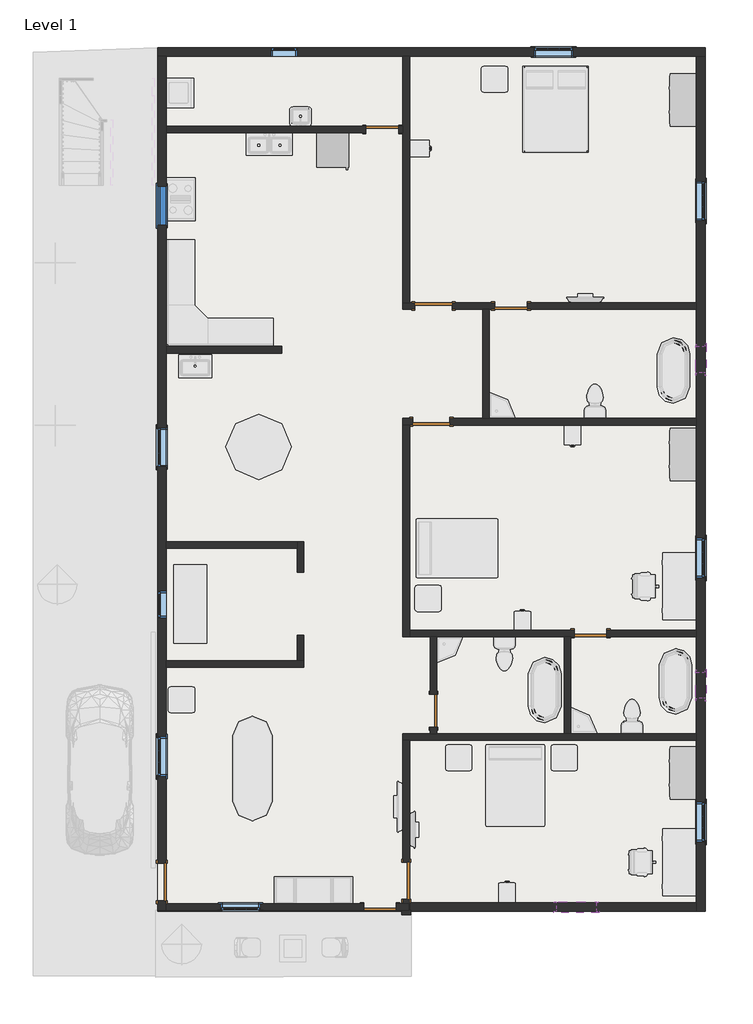
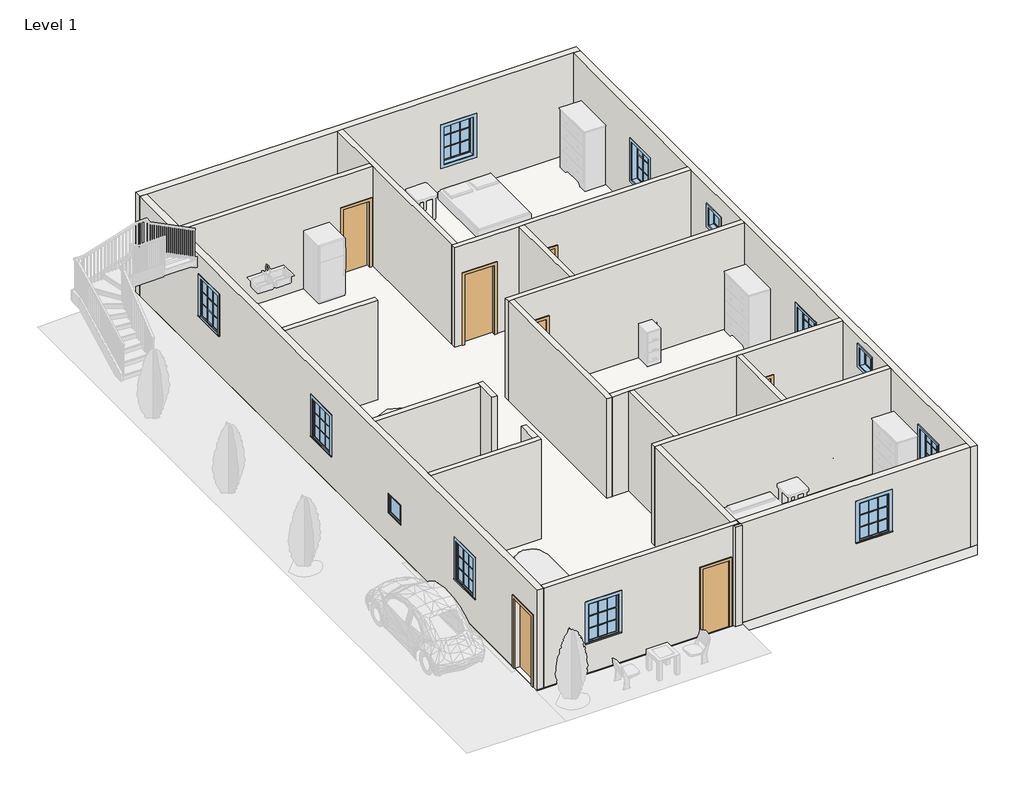
# One storey, part 1 of 3: 22 walls, 13 windows, 9 doors, 1 slab.
"""IFC4 building model written with IfcOpenShell, lengths in millimetres."""

from ifc_helpers import new_model, si_unit, frame, origin, origin_with_axes, place, context, project, spatial, polyline, outline, extrude, faceted_brep, transform, mapped, element, save
from components import door_059fdd7e, door_255cab33, door_99d96fc5, door_b6e9fca3, door_f75d31f8, window_29c06734, window_5c190c7e, window_6846e476, window_e41d21a6

model = new_model("IFC4")

# Units and contexts
model_context = context("Model", 3, world=origin())
ifc_project = project(units=[si_unit("LENGTHUNIT", "METRE", prefix="MILLI")], contexts=[model_context])

# Site, building, storey
site = spatial("IfcSite", under=ifc_project)
building = spatial("IfcBuilding", under=site)
storey = spatial("IfcBuildingStorey", under=building, Name="Level 1", Elevation=0.0)

# Doors
placement = place(None, origin())
door_shape = door_059fdd7e(model_context)
element("IfcDoor", 1, ObjectType="Single-Flush : 30\" x 80\"", at=placement, inside=storey, context=model_context, shape_type="MappedRepresentation", body=[
    mapped(door_shape, transform((-5854.9357228, 12907.8620171, 0.0), x_axis=(1.0, 0.0, 0.0), y_axis=(0.0, 1.0, 0.0), z_axis=(0.0, 0.0, 1.0))),
])
element("IfcDoor", 2, ObjectType="Single-Flush : 30\" x 80\"", at=placement, inside=storey, context=model_context, shape_type="MappedRepresentation", body=[
    mapped(door_shape, transform((-2857.7357228, 8793.0620171, 0.0), x_axis=(-1.0, 0.0, 0.0), y_axis=(0.0, -1.0, 0.0), z_axis=(0.0, 0.0, 1.0))),
])
element("IfcDoor", 3, ObjectType="Single-Flush : 30\" x 80\"", at=placement, inside=storey, context=model_context, shape_type="MappedRepresentation", body=[
    mapped(door_shape, transform((-4661.1357228, -630.3379829, 0.0), x_axis=(0.0, -1.0, 0.0), y_axis=(1.0, 0.0, 0.0), z_axis=(0.0, 0.0, 1.0))),
])
element("IfcDoor", 4, ObjectType="Single-Flush : 30\" x 80\"", at=placement, inside=storey, context=model_context, shape_type="MappedRepresentation", body=[
    mapped(door_shape, transform((-1003.5357228, 1173.0620171, 0.0), x_axis=(-1.0, 0.0, 0.0), y_axis=(0.0, -1.0, 0.0), z_axis=(0.0, 0.0, 1.0))),
])
door_2_shape = door_255cab33(model_context)
element("IfcDoor", 5, ObjectType="Single-Flush : 30\" x 80\"", at=placement, inside=storey, context=model_context, shape_type="MappedRepresentation", body=[
    mapped(door_2_shape, transform((-5905.7357228, -5202.3379829, 0.0), x_axis=(1.0, 0.0, 0.0), y_axis=(0.0, 1.0, 0.0), z_axis=(0.0, 0.0, 1.0))),
])
door_3_shape = door_99d96fc5(model_context)
element("IfcDoor", 6, ObjectType="Single-Flush : 34\" x 84\"", at=placement, inside=storey, context=model_context, shape_type="MappedRepresentation", body=[
    mapped(door_3_shape, transform((-4661.1357228, 8793.0620171, 0.0), x_axis=(-1.0, 0.0, 0.0), y_axis=(0.0, -1.0, 0.0), z_axis=(0.0, 0.0, 1.0))),
])
door_4_shape = door_b6e9fca3(model_context)
element("IfcDoor", 7, ObjectType="Single-Flush : 34\" x 84\"", at=placement, inside=storey, context=model_context, shape_type="MappedRepresentation", body=[
    mapped(door_4_shape, transform((-4711.9357228, 6100.6620171, 0.0), x_axis=(-1.0, 0.0, 0.0), y_axis=(0.0, -1.0, 0.0), z_axis=(0.0, 0.0, 1.0))),
])
element("IfcDoor", 8, ObjectType="Single-Flush : 34\" x 84\"", at=placement, inside=storey, context=model_context, shape_type="MappedRepresentation", body=[
    mapped(door_4_shape, transform((-5296.1357228, -4592.7379829, 0.0), x_axis=(0.0, -1.0, 0.0), y_axis=(1.0, 0.0, 0.0), z_axis=(0.0, 0.0, 1.0))),
])
door_5_shape = door_f75d31f8(model_context)
element("IfcDoor", 9, ObjectType="Single-Flush : 34\" x 84\"", at=placement, inside=storey, context=model_context, shape_type="MappedRepresentation", body=[
    mapped(door_5_shape, transform((-10985.7357228, -4618.1379829, 0.0), x_axis=(0.0, -1.0, 0.0), y_axis=(1.0, 0.0, 0.0), z_axis=(0.0, 0.0, 1.0))),
])

# Slab
element("IfcSlab", 10, ObjectType="Generic - 12\"", at=placement, inside=storey, context=model_context, shape_type="SweptSolid", body=[
    extrude(outline(polyline([(1663.4642772, 14812.8620171), (1663.4642772, -5227.7379829), (1663.4642772, -5303.9379829), (-11087.3357228, -5303.9379829), (-11087.3357228, 14812.8620171), (1663.4642772, 14812.8620171)])), frame((0.0, 0.0, -304.8), z_axis=(0.0, 0.0, 1.0), x_axis=(1.0, 0.0, 0.0)), (0.0, 0.0, 1.0), 304.8),
])

# Walls
element("IfcWall", 11, ObjectType="Generic - 8\"", at=placement, inside=storey, context=model_context, shape_type="Brep", body=[
    faceted_brep([(-11087.3357228, 14609.6620171, 0.0), (-10884.1357228, 14609.6620171, 0.0), (-5372.3357228, 14609.6620171, 0.0), (-5219.9357228, 14609.6620171, 0.0), (1460.2642772, 14609.6620171, 0.0), (1663.4642772, 14609.6620171, 0.0), (1663.4642772, 14609.6620171, 3048.0), (1460.2642772, 14609.6620171, 3048.0), (-5219.9357228, 14609.6620171, 3048.0), (-5372.3357228, 14609.6620171, 3048.0), (-10884.1357228, 14609.6620171, 3048.0), (-11087.3357228, 14609.6620171, 3048.0), (-1409.9357228, 14609.6620171, 2133.6), (-1409.9357228, 14609.6620171, 914.4), (-2324.3357228, 14609.6620171, 914.4), (-2324.3357228, 14609.6620171, 2133.6), (-7836.1357228, 14609.6620171, 1524.0), (-7836.1357228, 14609.6620171, 914.4), (-8445.7357228, 14609.6620171, 914.4), (-8445.7357228, 14609.6620171, 1524.0), (-11087.3357228, 14812.8620171, 0.0), (-11087.3357228, 14812.8620171, 3048.0), (1663.4642772, 14812.8620171, 3048.0), (1663.4642772, 14812.8620171, 0.0), (-1409.9357228, 14812.8620171, 2133.6), (-2324.3357228, 14812.8620171, 2133.6), (-2324.3357228, 14812.8620171, 914.4), (-1409.9357228, 14812.8620171, 914.4), (-7836.1357228, 14812.8620171, 1524.0), (-8445.7357228, 14812.8620171, 1524.0), (-8445.7357228, 14812.8620171, 914.4), (-7836.1357228, 14812.8620171, 914.4)], [[[0, 1, 2, 3, 4, 5, 6, 7, 8, 9, 10, 11], [12, 13, 14, 15], [16, 17, 18, 19]], [[20, 21, 22, 23], [24, 25, 26, 27], [28, 29, 30, 31]], [[5, 4, 3, 2, 1, 0, 20, 23]], [[6, 5, 23, 22]], [[0, 11, 21, 20]], [[13, 12, 24, 27]], [[14, 13, 27, 26]], [[15, 14, 26, 25]], [[12, 15, 25, 24]], [[17, 16, 28, 31]], [[18, 17, 31, 30]], [[19, 18, 30, 29]], [[16, 19, 29, 28]], [[11, 10, 9, 8, 7, 6, 22, 21]]]),
])
element("IfcWall", 12, ObjectType="Generic - 8\"", at=placement, inside=storey, context=model_context, shape_type="Brep", body=[
    faceted_brep([(1460.2642772, 14609.6620171, 0.0), (1460.2642772, 8869.2620171, 0.0), (1460.2642772, 8716.8620171, 0.0), (1460.2642772, 6176.8620171, 0.0), (1460.2642772, 6024.4620171, 0.0), (1460.2642772, 1249.2620171, 0.0), (1460.2642772, 1096.8620171, 0.0), (1460.2642772, -1163.7379829, 0.0), (1460.2642772, -1316.1379829, 0.0), (1460.2642772, -5100.7379829, 0.0), (1460.2642772, -5303.9379829, 0.0), (1460.2642772, -5303.9379829, 3048.0), (1460.2642772, -5100.7379829, 3048.0), (1460.2642772, -1316.1379829, 3048.0), (1460.2642772, -1163.7379829, 3048.0), (1460.2642772, 1096.8620171, 3048.0), (1460.2642772, 1249.2620171, 3048.0), (1460.2642772, 6024.4620171, 3048.0), (1460.2642772, 6176.8620171, 3048.0), (1460.2642772, 8716.8620171, 3048.0), (1460.2642772, 8869.2620171, 3048.0), (1460.2642772, 14609.6620171, 3048.0), (1460.2642772, 10786.9620171, 2133.6), (1460.2642772, 10786.9620171, 914.4), (1460.2642772, 11701.3620171, 914.4), (1460.2642772, 11701.3620171, 2133.6), (1460.2642772, 2468.4620171, 2133.6), (1460.2642772, 2468.4620171, 914.4), (1460.2642772, 3382.8620171, 914.4), (1460.2642772, 3382.8620171, 2133.6), (1460.2642772, -3678.3379829, 2133.6), (1460.2642772, -3678.3379829, 914.4), (1460.2642772, -2763.9379829, 914.4), (1460.2642772, -2763.9379829, 2133.6), (1460.2642772, 7243.6620171, 2463.8), (1460.2642772, 7243.6620171, 1854.2), (1460.2642772, 7853.2620171, 1854.2), (1460.2642772, 7853.2620171, 2463.8), (1460.2642772, -338.2379829, 2768.6), (1460.2642772, -338.2379829, 2159.0), (1460.2642772, 271.3620171, 2159.0), (1460.2642772, 271.3620171, 2768.6), (1663.4642772, 14609.6620171, 0.0), (1663.4642772, 14609.6620171, 3048.0), (1663.4642772, -5303.9379829, 3048.0), (1663.4642772, -5303.9379829, 0.0), (1663.4642772, 10786.9620171, 2133.6), (1663.4642772, 11701.3620171, 2133.6), (1663.4642772, 11701.3620171, 914.4), (1663.4642772, 10786.9620171, 914.4), (1663.4642772, 2468.4620171, 2133.6), (1663.4642772, 3382.8620171, 2133.6), (1663.4642772, 3382.8620171, 914.4), (1663.4642772, 2468.4620171, 914.4), (1663.4642772, -3678.3379829, 2133.6), (1663.4642772, -2763.9379829, 2133.6), (1663.4642772, -2763.9379829, 914.4), (1663.4642772, -3678.3379829, 914.4), (1663.4642772, 7243.6620171, 2463.8), (1663.4642772, 7853.2620171, 2463.8), (1663.4642772, 7853.2620171, 1854.2), (1663.4642772, 7243.6620171, 1854.2), (1663.4642772, -338.2379829, 2768.6), (1663.4642772, 271.3620171, 2768.6), (1663.4642772, 271.3620171, 2159.0), (1663.4642772, -338.2379829, 2159.0)], [[[0, 1, 2, 3, 4, 5, 6, 7, 8, 9, 10, 11, 12, 13, 14, 15, 16, 17, 18, 19, 20, 21], [22, 23, 24, 25], [26, 27, 28, 29], [30, 31, 32, 33], [34, 35, 36, 37], [38, 39, 40, 41]], [[42, 43, 44, 45], [46, 47, 48, 49], [50, 51, 52, 53], [54, 55, 56, 57], [58, 59, 60, 61], [62, 63, 64, 65]], [[10, 9, 8, 7, 6, 5, 4, 3, 2, 1, 0, 42, 45]], [[0, 21, 43, 42]], [[11, 10, 45, 44]], [[23, 22, 46, 49]], [[24, 23, 49, 48]], [[25, 24, 48, 47]], [[22, 25, 47, 46]], [[27, 26, 50, 53]], [[28, 27, 53, 52]], [[29, 28, 52, 51]], [[26, 29, 51, 50]], [[31, 30, 54, 57]], [[32, 31, 57, 56]], [[33, 32, 56, 55]], [[30, 33, 55, 54]], [[35, 34, 58, 61]], [[36, 35, 61, 60]], [[37, 36, 60, 59]], [[34, 37, 59, 58]], [[39, 38, 62, 65]], [[40, 39, 65, 64]], [[41, 40, 64, 63]], [[38, 41, 63, 62]], [[21, 20, 19, 18, 17, 16, 15, 14, 13, 12, 11, 44, 43]]]),
])
element("IfcWall", 13, ObjectType="Generic - 8\"", at=placement, inside=storey, context=model_context, shape_type="SweptSolid", body=[
    extrude(outline(polyline([(0.0, 1460.2642772), (3048.0, 1460.2642772), (3048.0, -5207.2357228), (0.0, -5207.2357228), (0.0, 1460.2642772)]), holes=[polyline([(2499.1543901, -1790.9357228), (2499.1543901, -876.5357228), (1279.9543901, -876.5357228), (1279.9543901, -1790.9357228), (2499.1543901, -1790.9357228)])]), frame((0.0, -5303.9379829, 0.0), z_axis=(0.0, 1.0, 0.0), x_axis=(0.0, 0.0, 1.0)), (0.0, 0.0, 1.0), 203.2),
])
element("IfcWall", 14, ObjectType="Generic - 8\"", at=placement, inside=storey, context=model_context, shape_type="Brep", body=[
    faceted_brep([(-5397.7357228, -5278.5379829, 0.0), (-5397.7357228, -5380.1379829, 0.0), (-5397.7357228, -5380.1379829, 3048.0), (-5397.7357228, -5303.9379829, 3048.0), (-5397.7357228, -5278.5379829, 3048.0), (-5194.5357228, -5278.5379829, 0.0), (-5194.5357228, -5278.5379829, 3048.0), (-5194.5357228, -5303.9379829, 3048.0), (-5194.5357228, -5380.1379829, 3048.0), (-5194.5357228, -5380.1379829, 0.0), (-5232.6357228, -5278.5379829, 0.0), (-5232.6357228, -5278.5379829, 3048.0)], [[[0, 1, 2, 3, 4]], [[5, 6, 7, 8, 9]], [[1, 0, 10, 5, 9]], [[2, 1, 9, 8]], [[0, 4, 11, 6, 5, 10]], [[3, 2, 8, 7]], [[4, 3, 7, 6, 11]]]),
])
element("IfcWall", 15, ObjectType="Generic - 8\"", at=placement, inside=storey, context=model_context, shape_type="Brep", body=[
    faceted_brep([(-10884.1357228, -5278.5379829, 0.0), (-10884.1357228, -5126.1379829, 0.0), (-10884.1357228, -5049.9379829, 0.0), (-10884.1357228, -5049.9379829, 2133.6), (-10884.1357228, -4186.3379829, 2133.6), (-10884.1357228, -4186.3379829, 0.0), (-10884.1357228, 385.6620171, 0.0), (-10884.1357228, 538.0620171, 0.0), (-10884.1357228, 3154.2620171, 0.0), (-10884.1357228, 3306.6620171, 0.0), (-10884.1357228, 7700.8620171, 0.0), (-10884.1357228, 7853.2620171, 0.0), (-10884.1357228, 12831.6620171, 0.0), (-10884.1357228, 12984.0620171, 0.0), (-10884.1357228, 14609.6620171, 0.0), (-10884.1357228, 14609.6620171, 3048.0), (-10884.1357228, 12984.0620171, 3048.0), (-10884.1357228, 12831.6620171, 3048.0), (-10884.1357228, 7853.2620171, 3048.0), (-10884.1357228, 7700.8620171, 3048.0), (-10884.1357228, 3306.6620171, 3048.0), (-10884.1357228, 3154.2620171, 3048.0), (-10884.1357228, 538.0620171, 3048.0), (-10884.1357228, 385.6620171, 3048.0), (-10884.1357228, -5126.1379829, 3048.0), (-10884.1357228, -5278.5379829, 3048.0), (-10884.1357228, -1239.9379829, 2133.6), (-10884.1357228, -1239.9379829, 914.4), (-10884.1357228, -2154.3379829, 914.4), (-10884.1357228, -2154.3379829, 2133.6), (-10884.1357228, 5960.9620171, 2133.6), (-10884.1357228, 5960.9620171, 914.4), (-10884.1357228, 5046.5620171, 914.4), (-10884.1357228, 5046.5620171, 2133.6), (-10884.1357228, 11587.0620171, 2413.0), (-10884.1357228, 11587.0620171, 1193.8), (-10884.1357228, 10672.6620171, 1193.8), (-10884.1357228, 10672.6620171, 2413.0), (-10884.1357228, 2150.9620171, 1524.0), (-10884.1357228, 2150.9620171, 914.4), (-10884.1357228, 1541.3620171, 914.4), (-10884.1357228, 1541.3620171, 1524.0), (-11087.3357228, -5049.9379829, 2133.6), (-11087.3357228, -5049.9379829, 0.0), (-11087.3357228, -5278.5379829, 0.0), (-11087.3357228, -5278.5379829, 3048.0), (-11087.3357228, 14609.6620171, 3048.0), (-11087.3357228, 14609.6620171, 0.0), (-11087.3357228, -4186.3379829, 0.0), (-11087.3357228, -4186.3379829, 2133.6), (-11087.3357228, -1239.9379829, 2133.6), (-11087.3357228, -2154.3379829, 2133.6), (-11087.3357228, -2154.3379829, 914.4), (-11087.3357228, -1239.9379829, 914.4), (-11087.3357228, 5960.9620171, 2133.6), (-11087.3357228, 5046.5620171, 2133.6), (-11087.3357228, 5046.5620171, 914.4), (-11087.3357228, 5960.9620171, 914.4), (-11087.3357228, 11587.0620171, 2413.0), (-11087.3357228, 10672.6620171, 2413.0), (-11087.3357228, 10672.6620171, 1193.8), (-11087.3357228, 11587.0620171, 1193.8), (-11087.3357228, 2150.9620171, 1524.0), (-11087.3357228, 1541.3620171, 1524.0), (-11087.3357228, 1541.3620171, 914.4), (-11087.3357228, 2150.9620171, 914.4)], [[[0, 1, 2, 3, 4, 5, 6, 7, 8, 9, 10, 11, 12, 13, 14, 15, 16, 17, 18, 19, 20, 21, 22, 23, 24, 25], [26, 27, 28, 29], [30, 31, 32, 33], [34, 35, 36, 37], [38, 39, 40, 41]], [[42, 43, 44, 45, 46, 47, 48, 49], [50, 51, 52, 53], [54, 55, 56, 57], [58, 59, 60, 61], [62, 63, 64, 65]], [[48, 47, 14, 13, 12, 11, 10, 9, 8, 7, 6, 5]], [[44, 43, 2, 1, 0]], [[15, 14, 47, 46]], [[5, 4, 49, 48]], [[4, 3, 42, 49]], [[3, 2, 43, 42]], [[26, 29, 51, 50]], [[29, 28, 52, 51]], [[28, 27, 53, 52]], [[27, 26, 50, 53]], [[30, 33, 55, 54]], [[33, 32, 56, 55]], [[32, 31, 57, 56]], [[31, 30, 54, 57]], [[34, 37, 59, 58]], [[37, 36, 60, 59]], [[36, 35, 61, 60]], [[35, 34, 58, 61]], [[38, 41, 63, 62]], [[41, 40, 64, 63]], [[40, 39, 65, 64]], [[39, 38, 62, 65]], [[0, 25, 45, 44]], [[25, 24, 23, 22, 21, 20, 19, 18, 17, 16, 15, 46, 45]]]),
])
element("IfcWall", 16, ObjectType="inner 6\"", at=placement, inside=storey, context=model_context, shape_type="Brep", body=[
    faceted_brep([(-5372.3357228, 14609.6620171, 0.0), (-5372.3357228, 12984.0620171, 0.0), (-5372.3357228, 12831.6620171, 0.0), (-5372.3357228, 8869.2620171, 0.0), (-5372.3357228, 8869.2620171, 3048.0), (-5372.3357228, 12831.6620171, 3048.0), (-5372.3357228, 12984.0620171, 3048.0), (-5372.3357228, 14609.6620171, 3048.0), (-5219.9357228, 14609.6620171, 0.0), (-5219.9357228, 14609.6620171, 3048.0), (-5219.9357228, 8869.2620171, 3048.0), (-5219.9357228, 8869.2620171, 0.0)], [[[0, 1, 2, 3, 4, 5, 6, 7]], [[8, 9, 10, 11]], [[3, 2, 1, 0, 8, 11]], [[0, 7, 9, 8]], [[4, 3, 11, 10]], [[7, 6, 5, 4, 10, 9]]]),
])
element("IfcWall", 17, ObjectType="inner 6\"", at=placement, inside=storey, context=model_context, shape_type="Brep", body=[
    faceted_brep([(-3238.7357228, 8869.2620171, 2032.0), (-3238.7357228, 8869.2620171, 0.0), (-4229.3357228, 8869.2620171, 0.0), (-4229.3357228, 8869.2620171, 2133.6), (-5092.9357228, 8869.2620171, 2133.6), (-5092.9357228, 8869.2620171, 0.0), (-5219.9357228, 8869.2620171, 0.0), (-5372.3357228, 8869.2620171, 0.0), (-5372.3357228, 8869.2620171, 3048.0), (-5219.9357228, 8869.2620171, 3048.0), (1460.2642772, 8869.2620171, 3048.0), (1460.2642772, 8869.2620171, 0.0), (-2476.7357228, 8869.2620171, 0.0), (-2476.7357228, 8869.2620171, 2032.0), (-4229.3357228, 8716.8620171, 0.0), (-3518.1357228, 8716.8620171, 0.0), (-3365.7357228, 8716.8620171, 0.0), (-3238.7357228, 8716.8620171, 0.0), (-3238.7357228, 8716.8620171, 2032.0), (-2476.7357228, 8716.8620171, 2032.0), (-2476.7357228, 8716.8620171, 0.0), (1460.2642772, 8716.8620171, 0.0), (1460.2642772, 8716.8620171, 3048.0), (-3365.7357228, 8716.8620171, 3048.0), (-3518.1357228, 8716.8620171, 3048.0), (-5372.3357228, 8716.8620171, 3048.0), (-5372.3357228, 8716.8620171, 0.0), (-5092.9357228, 8716.8620171, 0.0), (-5092.9357228, 8716.8620171, 2133.6), (-4229.3357228, 8716.8620171, 2133.6)], [[[0, 1, 2, 3, 4, 5, 6, 7, 8, 9, 10, 11, 12, 13]], [[14, 15, 16, 17, 18, 19, 20, 21, 22, 23, 24, 25, 26, 27, 28, 29]], [[7, 6, 5, 27, 26]], [[12, 11, 21, 20]], [[2, 1, 17, 16, 15, 14]], [[11, 10, 22, 21]], [[8, 7, 26, 25]], [[28, 27, 5, 4]], [[29, 28, 4, 3]], [[14, 29, 3, 2]], [[18, 17, 1, 0]], [[19, 18, 0, 13]], [[20, 19, 13, 12]], [[10, 9, 8, 25, 24, 23, 22]]]),
])
element("IfcWall", 18, ObjectType="inner 6\"", at=placement, inside=storey, context=model_context, shape_type="SweptSolid", body=[
    extrude(outline(polyline([(-3518.1357228, 6176.8620171), (-3518.1357228, 8716.8620171), (-3365.7357228, 8716.8620171), (-3365.7357228, 6176.8620171), (-3518.1357228, 6176.8620171)])), origin_with_axes(), (0.0, 0.0, 1.0), 3048.0),
])
element("IfcWall", 19, ObjectType="inner 6\"", at=placement, inside=storey, context=model_context, shape_type="Brep", body=[
    faceted_brep([(-5372.3357228, 6024.4620171, 0.0), (-5219.9357228, 6024.4620171, 0.0), (-5143.7357228, 6024.4620171, 0.0), (-5143.7357228, 6024.4620171, 2133.6), (-4280.1357228, 6024.4620171, 2133.6), (-4280.1357228, 6024.4620171, 0.0), (1460.2642772, 6024.4620171, 0.0), (1460.2642772, 6024.4620171, 3048.0), (-5219.9357228, 6024.4620171, 3048.0), (-5372.3357228, 6024.4620171, 3048.0), (-5143.7357228, 6176.8620171, 2133.6), (-5143.7357228, 6176.8620171, 0.0), (-5372.3357228, 6176.8620171, 0.0), (-5372.3357228, 6176.8620171, 3048.0), (-3518.1357228, 6176.8620171, 3048.0), (-3365.7357228, 6176.8620171, 3048.0), (1460.2642772, 6176.8620171, 3048.0), (1460.2642772, 6176.8620171, 0.0), (-3365.7357228, 6176.8620171, 0.0), (-3518.1357228, 6176.8620171, 0.0), (-4280.1357228, 6176.8620171, 0.0), (-4280.1357228, 6176.8620171, 2133.6)], [[[0, 1, 2, 3, 4, 5, 6, 7, 8, 9]], [[10, 11, 12, 13, 14, 15, 16, 17, 18, 19, 20, 21]], [[12, 11, 2, 1, 0]], [[20, 19, 18, 17, 6, 5]], [[7, 6, 17, 16]], [[0, 9, 13, 12]], [[3, 2, 11, 10]], [[4, 3, 10, 21]], [[5, 4, 21, 20]], [[9, 8, 7, 16, 15, 14, 13]]]),
])
element("IfcWall", 20, ObjectType="inner 6\"", at=placement, inside=storey, context=model_context, shape_type="Brep", body=[
    faceted_brep([(-5372.3357228, 6024.4620171, 0.0), (-5372.3357228, 1096.8620171, 0.0), (-5372.3357228, 1096.8620171, 3048.0), (-5372.3357228, 6024.4620171, 3048.0), (-5219.9357228, 6024.4620171, 0.0), (-5219.9357228, 6024.4620171, 3048.0), (-5219.9357228, 1249.2620171, 3048.0), (-5219.9357228, 1096.8620171, 3048.0), (-5219.9357228, 1096.8620171, 0.0), (-5219.9357228, 1249.2620171, 0.0)], [[[0, 1, 2, 3]], [[4, 5, 6, 7, 8, 9]], [[1, 0, 4, 9, 8]], [[0, 3, 5, 4]], [[2, 1, 8, 7]], [[3, 2, 7, 6, 5]]]),
])
element("IfcWall", 21, ObjectType="inner 6\"", at=placement, inside=storey, context=model_context, shape_type="Brep", body=[
    faceted_brep([(-5219.9357228, 1096.8620171, 0.0), (-4737.3357228, 1096.8620171, 0.0), (-4584.9357228, 1096.8620171, 0.0), (-1613.1357228, 1096.8620171, 0.0), (-1460.7357228, 1096.8620171, 0.0), (-1384.5357228, 1096.8620171, 0.0), (-1384.5357228, 1096.8620171, 2032.0), (-622.5357228, 1096.8620171, 2032.0), (-622.5357228, 1096.8620171, 0.0), (1460.2642772, 1096.8620171, 0.0), (1460.2642772, 1096.8620171, 3048.0), (-1460.7357228, 1096.8620171, 3048.0), (-1613.1357228, 1096.8620171, 3048.0), (-4584.9357228, 1096.8620171, 3048.0), (-4737.3357228, 1096.8620171, 3048.0), (-5219.9357228, 1096.8620171, 3048.0), (-1384.5357228, 1249.2620171, 2032.0), (-1384.5357228, 1249.2620171, 0.0), (-5219.9357228, 1249.2620171, 0.0), (-5219.9357228, 1249.2620171, 3048.0), (1460.2642772, 1249.2620171, 3048.0), (1460.2642772, 1249.2620171, 0.0), (-622.5357228, 1249.2620171, 0.0), (-622.5357228, 1249.2620171, 2032.0)], [[[0, 1, 2, 3, 4, 5, 6, 7, 8, 9, 10, 11, 12, 13, 14, 15]], [[16, 17, 18, 19, 20, 21, 22, 23]], [[22, 21, 9, 8]], [[18, 17, 5, 4, 3, 2, 1, 0]], [[0, 15, 19, 18]], [[10, 9, 21, 20]], [[6, 5, 17, 16]], [[7, 6, 16, 23]], [[8, 7, 23, 22]], [[15, 14, 13, 12, 11, 10, 20, 19]]]),
])
element("IfcWall", 22, ObjectType="inner 6\"", at=placement, inside=storey, context=model_context, shape_type="Brep", body=[
    faceted_brep([(-5372.3357228, -1316.1379829, 0.0), (-5219.9357228, -1316.1379829, 0.0), (1460.2642772, -1316.1379829, 0.0), (1460.2642772, -1316.1379829, 3048.0), (-5219.9357228, -1316.1379829, 3048.0), (-5372.3357228, -1316.1379829, 3048.0), (-5372.3357228, -1163.7379829, 0.0), (-5372.3357228, -1163.7379829, 3048.0), (-4737.3357228, -1163.7379829, 3048.0), (-4584.9357228, -1163.7379829, 3048.0), (-1613.1357228, -1163.7379829, 3048.0), (-1460.7357228, -1163.7379829, 3048.0), (1460.2642772, -1163.7379829, 3048.0), (1460.2642772, -1163.7379829, 0.0), (-1460.7357228, -1163.7379829, 0.0), (-1613.1357228, -1163.7379829, 0.0), (-4584.9357228, -1163.7379829, 0.0), (-4737.3357228, -1163.7379829, 0.0)], [[[0, 1, 2, 3, 4, 5]], [[6, 7, 8, 9, 10, 11, 12, 13, 14, 15, 16, 17]], [[2, 1, 0, 6, 17, 16, 15, 14, 13]], [[3, 2, 13, 12]], [[0, 5, 7, 6]], [[5, 4, 3, 12, 11, 10, 9, 8, 7]]]),
])
element("IfcWall", 23, ObjectType="inner 6\"", at=placement, inside=storey, context=model_context, shape_type="SweptSolid", body=[
    extrude(outline(polyline([(-1011.3379829, 2032.0), (-1011.3379829, 0.0), (-1163.7379829, 0.0), (-1163.7379829, 3048.0), (1096.8620171, 3048.0), (1096.8620171, 0.0), (-249.3379829, 0.0), (-249.3379829, 2032.0), (-1011.3379829, 2032.0)])), frame((-4737.3357228, 0.0, 0.0), z_axis=(1.0, 0.0, 0.0), x_axis=(0.0, 1.0, 0.0)), (0.0, 0.0, 1.0), 152.4),
])
element("IfcWall", 24, ObjectType="inner 6\"", at=placement, inside=storey, context=model_context, shape_type="SweptSolid", body=[
    extrude(outline(polyline([(-1613.1357228, -1163.7379829), (-1613.1357228, 1096.8620171), (-1460.7357228, 1096.8620171), (-1460.7357228, -1163.7379829), (-1613.1357228, -1163.7379829)])), origin_with_axes(), (0.0, 0.0, 1.0), 3048.0),
])
element("IfcWall", 25, ObjectType="inner 6\"", at=placement, inside=storey, context=model_context, shape_type="Brep", body=[
    faceted_brep([(-5372.3357228, -5024.5379829, 2133.6), (-5372.3357228, -5024.5379829, 0.0), (-5372.3357228, -5126.1379829, 0.0), (-5372.3357228, -5126.1379829, 3048.0), (-5372.3357228, -1316.1379829, 3048.0), (-5372.3357228, -1316.1379829, 0.0), (-5372.3357228, -4160.9379829, 0.0), (-5372.3357228, -4160.9379829, 2133.6), (-5219.9357228, -5126.1379829, 0.0), (-5219.9357228, -5024.5379829, 0.0), (-5219.9357228, -5024.5379829, 2133.6), (-5219.9357228, -4160.9379829, 2133.6), (-5219.9357228, -4160.9379829, 0.0), (-5219.9357228, -1316.1379829, 0.0), (-5219.9357228, -1316.1379829, 3048.0), (-5219.9357228, -5126.1379829, 3048.0), (-5232.6357228, -5126.1379829, 0.0), (-5232.6357228, -5126.1379829, 3048.0)], [[[0, 1, 2, 3, 4, 5, 6, 7]], [[8, 9, 10, 11, 12, 13, 14, 15]], [[6, 5, 13, 12]], [[2, 1, 9, 8, 16]], [[5, 4, 14, 13]], [[3, 2, 16, 8, 15, 17]], [[10, 9, 1, 0]], [[11, 10, 0, 7]], [[12, 11, 7, 6]], [[4, 3, 17, 15, 14]]]),
])
element("IfcWall", 26, ObjectType="inner 6\"", at=placement, inside=storey, context=model_context, shape_type="Brep", body=[
    faceted_brep([(-10884.1357228, 385.6620171, 0.0), (-7683.7357228, 385.6620171, 0.0), (-7683.7357228, 385.6620171, 3048.0), (-10884.1357228, 385.6620171, 3048.0), (-10884.1357228, 538.0620171, 0.0), (-10884.1357228, 538.0620171, 3048.0), (-7836.1357228, 538.0620171, 3048.0), (-7683.7357228, 538.0620171, 3048.0), (-7683.7357228, 538.0620171, 0.0), (-7836.1357228, 538.0620171, 0.0)], [[[0, 1, 2, 3]], [[4, 5, 6, 7, 8, 9]], [[1, 0, 4, 9, 8]], [[0, 3, 5, 4]], [[2, 1, 8, 7]], [[3, 2, 7, 6, 5]]]),
])
element("IfcWall", 27, ObjectType="inner 6\"", at=placement, inside=storey, context=model_context, shape_type="SweptSolid", body=[
    extrude(outline(polyline([(-7683.7357228, 1122.2620171), (-7683.7357228, 538.0620171), (-7836.1357228, 538.0620171), (-7836.1357228, 1122.2620171), (-7683.7357228, 1122.2620171)])), origin_with_axes(), (0.0, 0.0, 1.0), 3048.0),
])
element("IfcWall", 28, ObjectType="inner 6\"", at=placement, inside=storey, context=model_context, shape_type="SweptSolid", body=[
    extrude(outline(polyline([(-10884.1357228, 3306.6620171), (-7836.1357228, 3306.6620171), (-7836.1357228, 3154.2620171), (-10884.1357228, 3154.2620171), (-10884.1357228, 3306.6620171)])), origin_with_axes(), (0.0, 0.0, 1.0), 3048.0),
])
element("IfcWall", 29, ObjectType="inner 6\"", at=placement, inside=storey, context=model_context, shape_type="Brep", body=[
    faceted_brep([(-5232.6357228, -5126.1379829, 0.0), (-5372.3357228, -5126.1379829, 0.0), (-5524.7357228, -5126.1379829, 0.0), (-5524.7357228, -5126.1379829, 2032.0), (-6286.7357228, -5126.1379829, 2032.0), (-6286.7357228, -5126.1379829, 0.0), (-10884.1357228, -5126.1379829, 0.0), (-10884.1357228, -5126.1379829, 3048.0), (-5372.3357228, -5126.1379829, 3048.0), (-5232.6357228, -5126.1379829, 3048.0), (-9614.1357228, -5126.1379829, 2133.6), (-9614.1357228, -5126.1379829, 914.4), (-8699.7357228, -5126.1379829, 914.4), (-8699.7357228, -5126.1379829, 2133.6), (-5524.7357228, -5278.5379829, 2032.0), (-5524.7357228, -5278.5379829, 0.0), (-5397.7357228, -5278.5379829, 0.0), (-5232.6357228, -5278.5379829, 0.0), (-5232.6357228, -5278.5379829, 3048.0), (-5397.7357228, -5278.5379829, 3048.0), (-10884.1357228, -5278.5379829, 3048.0), (-10884.1357228, -5278.5379829, 0.0), (-6286.7357228, -5278.5379829, 0.0), (-6286.7357228, -5278.5379829, 2032.0), (-9614.1357228, -5278.5379829, 2133.6), (-8699.7357228, -5278.5379829, 2133.6), (-8699.7357228, -5278.5379829, 914.4), (-9614.1357228, -5278.5379829, 914.4)], [[[0, 1, 2, 3, 4, 5, 6, 7, 8, 9], [10, 11, 12, 13]], [[14, 15, 16, 17, 18, 19, 20, 21, 22, 23], [24, 25, 26, 27]], [[22, 21, 6, 5]], [[17, 16, 15, 2, 1, 0]], [[0, 9, 18, 17]], [[7, 6, 21, 20]], [[3, 2, 15, 14]], [[4, 3, 14, 23]], [[5, 4, 23, 22]], [[11, 10, 24, 27]], [[12, 11, 27, 26]], [[13, 12, 26, 25]], [[10, 13, 25, 24]], [[9, 8, 7, 20, 19, 18]]]),
])
element("IfcWall", 30, ObjectType="inner 6\"", at=placement, inside=storey, context=model_context, shape_type="SweptSolid", body=[
    extrude(outline(polyline([(2032.0, -5473.9357228), (0.0, -5473.9357228), (0.0, -5372.3357228), (3048.0, -5372.3357228), (3048.0, -10884.1357228), (0.0, -10884.1357228), (0.0, -6235.9357228), (2032.0, -6235.9357228), (2032.0, -5473.9357228)])), frame((0.0, 12831.6620171, 0.0), z_axis=(0.0, 1.0, 0.0), x_axis=(0.0, 0.0, 1.0)), (0.0, 0.0, 1.0), 152.4),
])
element("IfcWall", 31, ObjectType="inner 6\"", at=placement, inside=storey, context=model_context, shape_type="SweptSolid", body=[
    extrude(outline(polyline([(-10884.1357228, 7853.2620171), (-8191.7357228, 7853.2620171), (-8191.7357228, 7700.8620171), (-10884.1357228, 7700.8620171), (-10884.1357228, 7853.2620171)])), origin_with_axes(), (0.0, 0.0, 1.0), 3048.0),
])
element("IfcWall", 32, ObjectType="inner 6\"", at=placement, inside=storey, context=model_context, shape_type="Brep", body=[
    faceted_brep([(-7683.7357228, 2595.4620171, 0.0), (-7683.7357228, 3306.6620171, 0.0), (-7683.7357228, 3306.6620171, 3048.0), (-7683.7357228, 2595.4620171, 3048.0), (-7836.1357228, 2595.4620171, 0.0), (-7836.1357228, 2595.4620171, 3048.0), (-7836.1357228, 3154.2620171, 3048.0), (-7836.1357228, 3306.6620171, 3048.0), (-7836.1357228, 3306.6620171, 0.0), (-7836.1357228, 3154.2620171, 0.0)], [[[0, 1, 2, 3]], [[4, 5, 6, 7, 8, 9]], [[1, 0, 4, 9, 8]], [[0, 3, 5, 4]], [[2, 1, 8, 7]], [[3, 2, 7, 6, 5]]]),
])

# Windows
window_shape = window_29c06734(model_context)
element("IfcWindow", 33, ObjectType="Casement 3x3 with Trim : 36\" x 48\"", at=placement, inside=storey, context=model_context, shape_type="MappedRepresentation", body=[
    mapped(window_shape, transform((-1867.1357228, 14711.2620171, 0.0), x_axis=(1.0, 0.0, 0.0), y_axis=(0.0, 1.0, 0.0), z_axis=(0.0, 0.0, 1.0))),
])
element("IfcWindow", 34, ObjectType="Casement 3x3 with Trim : 36\" x 48\"", at=placement, inside=storey, context=model_context, shape_type="MappedRepresentation", body=[
    mapped(window_shape, transform((1561.8642772, 11244.1620171, 0.0), x_axis=(0.0, -1.0, 0.0), y_axis=(1.0, 0.0, 0.0), z_axis=(0.0, 0.0, 1.0))),
])
element("IfcWindow", 35, ObjectType="Casement 3x3 with Trim : 36\" x 48\"", at=placement, inside=storey, context=model_context, shape_type="MappedRepresentation", body=[
    mapped(window_shape, transform((1561.8642772, 2925.6620171, 0.0), x_axis=(0.0, -1.0, 0.0), y_axis=(1.0, 0.0, 0.0), z_axis=(0.0, 0.0, 1.0))),
])
element("IfcWindow", 36, ObjectType="Casement 3x3 with Trim : 36\" x 48\"", at=placement, inside=storey, context=model_context, shape_type="MappedRepresentation", body=[
    mapped(window_shape, transform((1561.8642772, -3221.1379829, 0.0), x_axis=(0.0, -1.0, 0.0), y_axis=(1.0, 0.0, 0.0), z_axis=(0.0, 0.0, 1.0))),
])
element("IfcWindow", 37, ObjectType="Casement 3x3 with Trim : 36\" x 48\"", at=placement, inside=storey, context=model_context, shape_type="MappedRepresentation", body=[
    mapped(window_shape, transform((-10985.7357228, -1697.1379829, 0.0), x_axis=(0.0, 1.0, 0.0), y_axis=(-1.0, 0.0, 0.0), z_axis=(0.0, 0.0, 1.0))),
])
element("IfcWindow", 38, ObjectType="Casement 3x3 with Trim : 36\" x 48\"", at=placement, inside=storey, context=model_context, shape_type="MappedRepresentation", body=[
    mapped(window_shape, transform((-10985.7357228, 5503.7620171, 0.0), x_axis=(0.0, 1.0, 0.0), y_axis=(-1.0, 0.0, 0.0), z_axis=(0.0, 0.0, 1.0))),
])
element("IfcWindow", 39, ObjectType="Casement 3x3 with Trim : 36\" x 48\"", at=placement, inside=storey, context=model_context, shape_type="MappedRepresentation", body=[
    mapped(window_shape, transform((-10985.7357228, 11129.8620171, 279.4), x_axis=(0.0, 1.0, 0.0), y_axis=(-1.0, 0.0, 0.0), z_axis=(0.0, 0.0, 1.0))),
])
element("IfcWindow", 40, ObjectType="Casement 3x3 with Trim : 36\" x 48\"", at=placement, inside=storey, context=model_context, shape_type="MappedRepresentation", body=[
    mapped(window_shape, transform((-1333.7357228, -5202.3379829, 365.5543901), x_axis=(-1.0, 0.0, 0.0), y_axis=(0.0, -1.0, 0.0), z_axis=(0.0, 0.0, 1.0))),
])
window_2_shape = window_5c190c7e(model_context)
element("IfcWindow", 41, ObjectType="Casement 3x3 with Trim : 36\" x 48\"", at=placement, inside=storey, context=model_context, shape_type="MappedRepresentation", body=[
    mapped(window_2_shape, transform((-9156.9357228, -5202.3379829, 0.0), x_axis=(-1.0, 0.0, 0.0), y_axis=(0.0, -1.0, 0.0), z_axis=(0.0, 0.0, 1.0))),
])
window_3_shape = window_6846e476(model_context)
element("IfcWindow", 42, ObjectType="Fixed : 24\" x 24\"", at=placement, inside=storey, context=model_context, shape_type="MappedRepresentation", body=[
    mapped(window_3_shape, transform((-10985.7357228, 1884.2620171, 0.0), x_axis=(0.0, 1.0, 0.0), y_axis=(-1.0, 0.0, 0.0), z_axis=(0.0, 0.0, 1.0))),
])
element("IfcWindow", 43, ObjectType="Fixed : 24\" x 24\"", at=placement, inside=storey, context=model_context, shape_type="MappedRepresentation", body=[
    mapped(window_3_shape, transform((-8102.8357228, 14711.2620171, 0.0), x_axis=(1.0, 0.0, 0.0), y_axis=(0.0, 1.0, 0.0), z_axis=(0.0, 0.0, 1.0))),
])
window_4_shape = window_e41d21a6(model_context)
element("IfcWindow", 44, ObjectType="Transom with Trim : 24\" x 24\"", at=placement, inside=storey, context=model_context, shape_type="MappedRepresentation", body=[
    mapped(window_4_shape, transform((1561.8642772, 7510.3620171, -304.8), x_axis=(0.0, -1.0, 0.0), y_axis=(1.0, 0.0, 0.0), z_axis=(0.0, 0.0, 1.0))),
])
element("IfcWindow", 45, ObjectType="Transom with Trim : 24\" x 24\"", at=placement, inside=storey, context=model_context, shape_type="MappedRepresentation", body=[
    mapped(window_4_shape, transform((1561.8642772, -71.5379829, 0.0), x_axis=(0.0, -1.0, 0.0), y_axis=(1.0, 0.0, 0.0), z_axis=(0.0, 0.0, 1.0))),
])

save(model, "model.ifc")

# Revit data of these elements
# Type "Single-Flush : 30\" x 80\""
#   Type Mark = "5"
#   Construction Type Id = "MDOOR"
#   Assembly Code = "C1020"
#   Analytic Construction = "Metal"
#   Thickness = 0' - 2"
#   Heat Transfer Coefficient (U) = 0.651978 BTU/(h·ft²·°F)
#   Height = 6' - 8"
#   Trim Projection Ext = 0' - 1"
#   Trim Projection Int = 0' - 1"
#   Trim Width = 0' - 3"
#   Width = 2' - 6"
#   Define Thermal Properties by = 1
#   Door Material = Door - Panel
#   Frame Material = Door - Frame
#   Visual Light Transmittance = 0
#   Solar Heat Gain Coefficient = 0
#   Function = (empty or 0)
#   Wall Closure = (empty or 0)
# Type "Single-Flush : 34\" x 84\""
#   Type Mark = "2"
#   Construction Type Id = "MDOOR"
#   Assembly Code = "C1020"
#   Analytic Construction = "Metal"
#   Thickness = 0' - 2"
#   Heat Transfer Coefficient (U) = 0.651978 BTU/(h·ft²·°F)
#   Height = 7' - 0"
#   Trim Projection Ext = 0' - 1"
#   Trim Projection Int = 0' - 1"
#   Trim Width = 0' - 3"
#   Width = 2' - 10"
#   Define Thermal Properties by = 1
#   Door Material = Door - Panel
#   Frame Material = Door - Frame
#   Visual Light Transmittance = 0
#   Solar Heat Gain Coefficient = 0
#   Function = (empty or 0)
#   Wall Closure = (empty or 0)
# Type "Generic - 12\""
#   Assembly Code = "B1010"
#   Function = 0
#   Layers, outside or top first: 1' - 0" no material (function 1)
# Type "Generic - 8\""
#   Assembly Code = "B2010"
#   Layers, outside or top first: 0' - 8" "Brick, Common" (function 1)
# Type "inner 6\""
#   Assembly Code = "B2010"
#   Layers, outside or top first: 0' - 6" "Brick, Common" (function 1)
# Type "Casement 3x3 with Trim : 36\" x 48\""
#   Type Mark = "10"
#   Construction Type Id = "GSP4R"
#   Assembly Code = "B2020100"
#   Analytic Construction = "1/8 in Pilkington single glazing"
#   Visual Light Transmittance = 0.9
#   Solar Heat Gain Coefficient = 0.78
#   Heat Transfer Coefficient (U) = 0.6496 BTU/(h·ft²·°F)
#   Height = 4' - 0"
#   Default Sill Height = 3' - 0"
#   Trim Projection - Ext. = 0' - 0 1/2"
#   Trim Projection - Int. = 0' - 0 3/4"
#   Trim Width - Exterior = 0' - 3 1/2"
#   Trim Width - Interior = 0' - 3 1/2"
#   Width = 3' - 0"
#   Window Inset = 0' - 0 3/4"
#   Define Thermal Properties by = 1
#   Glass Pane Material = Glass
#   Sash Material = Sash
#   Trim Exterior Material = Trim
#   Trim Interior Material = Trim
#   Wall Closure = (empty or 0)
# Type "Fixed : 24\" x 24\""
#   Type Mark = "3"
#   Construction Type Id = "GSP4R"
#   Assembly Code = "B2020100"
#   Analytic Construction = "1/8 in Pilkington single glazing"
#   Visual Light Transmittance = 0.9
#   Solar Heat Gain Coefficient = 0.78
#   Heat Transfer Coefficient (U) = 0.6496 BTU/(h·ft²·°F)
#   Height = 2' - 0"
#   Default Sill Height = 3' - 0"
#   Width = 2' - 0"
#   Window Inset = 0' - 0 3/4"
#   Define Thermal Properties by = 1
#   Glass Pane Material = Glass
#   Sash Material = Sash
#   Wall Closure = (empty or 0)
# Type "Transom with Trim : 24\" x 24\""
#   Type Mark = "13"
#   Construction Type Id = "GSP4R"
#   Assembly Code = "B2020100"
#   Analytic Construction = "1/8 in Pilkington single glazing"
#   Visual Light Transmittance = 0.9
#   Solar Heat Gain Coefficient = 0.78
#   Heat Transfer Coefficient (U) = 0.6496 BTU/(h·ft²·°F)
#   Height = 2' - 0"
#   Default Sill Height = 7' - 1"
#   Trim Projection - Ext. = 0' - 0 1/2"
#   Trim Projection - Int. = 0' - 0 3/4"
#   Trim Width - Exterior = 0' - 3 1/2"
#   Trim Width - Interior = 0' - 3 1/2"
#   Width = 2' - 0"
#   Window Inset = 0' - 0 3/4"
#   Define Thermal Properties by = 1
#   Glass Pane Material = Glass
#   Sash Material = Sash
#   Trim Exterior Material = Trim
#   Trim Interior Material = Trim
#   Wall Closure = (empty or 0)
# Elements 1, 2, 3, 4, 5 (IfcDoor, "Single-Flush : 30\" x 80\"")
#   Phase Created = New Construction
#   Materials on its faces: "Door - Frame", "Door - Panel"
# Elements 6, 7, 8, 9 (IfcDoor, "Single-Flush : 34\" x 84\"")
#   Phase Created = New Construction
#   Materials on its faces: "Door - Frame", "Door - Panel"
# Element 10 (IfcSlab, "Generic - 12\"")
#   Height Offset From Level = 0' - 0"
#   Phase Created = New Construction
#   Materials on its faces: "Default Floor"
# Elements 11, 12, 13, 14, 15 (IfcWall, "Generic - 8\"")
#   Top Offset = 0' - 0"
#   Base Offset = 0' - 0"
#   Unconnected Height = 10' - 0"
#   wall height = 10' - 0"
#   Phase Created = New Construction
#   Base Constraint = Level 1
#   Materials on its faces: "Brick, Common"
# Elements 16, 17, 18, 19, 20, 21, 22, 23, 24, 25, 26, 27, 28, 29, 30, 31, 32 (IfcWall, "inner 6\"")
#   Top Offset = 0' - 0"
#   Base Offset = 0' - 0"
#   Unconnected Height = 10' - 0"
#   wall height = 10' - 0"
#   Phase Created = New Construction
#   Base Constraint = Level 1
#   Materials on its faces: "Brick, Common"
# Element 33 (IfcWindow, "Casement 3x3 with Trim : 36\" x 48\"")
#   Mark = "1"
#   Phase Created = New Construction
#   Materials on its faces: "Sash", "Glass", "Trim"
# Element 34 (IfcWindow, "Casement 3x3 with Trim : 36\" x 48\"")
#   Mark = "2"
#   Phase Created = New Construction
#   Materials on its faces: "Sash", "Glass", "Trim"
# Element 35 (IfcWindow, "Casement 3x3 with Trim : 36\" x 48\"")
#   Mark = "3"
#   Phase Created = New Construction
#   Materials on its faces: "Sash", "Glass", "Trim"
# Element 36 (IfcWindow, "Casement 3x3 with Trim : 36\" x 48\"")
#   Mark = "4"
#   Phase Created = New Construction
#   Materials on its faces: "Sash", "Glass", "Trim"
# Element 37 (IfcWindow, "Casement 3x3 with Trim : 36\" x 48\"")
#   Mark = "6"
#   Phase Created = New Construction
#   Materials on its faces: "Sash", "Glass", "Trim"
# Element 38 (IfcWindow, "Casement 3x3 with Trim : 36\" x 48\"")
#   Mark = "7"
#   Phase Created = New Construction
#   Materials on its faces: "Sash", "Glass", "Trim"
# Element 39 (IfcWindow, "Casement 3x3 with Trim : 36\" x 48\"")
#   Mark = "8"
#   Phase Created = New Construction
#   Materials on its faces: "Sash", "Glass", "Trim"
# Element 40 (IfcWindow, "Casement 3x3 with Trim : 36\" x 48\"")
#   Mark = "13"
#   Phase Created = New Construction
#   Materials on its faces: "Sash", "Glass", "Trim"
# Element 41 (IfcWindow, "Casement 3x3 with Trim : 36\" x 48\"")
#   Mark = "5"
#   Phase Created = New Construction
#   Materials on its faces: "Sash", "Glass", "Trim"
# Element 42 (IfcWindow, "Fixed : 24\" x 24\"")
#   Mark = "11"
#   Phase Created = New Construction
#   Materials on its faces: "Sash", "Glass"
# Element 43 (IfcWindow, "Fixed : 24\" x 24\"")
#   Mark = "12"
#   Phase Created = New Construction
#   Materials on its faces: "Sash", "Glass"
# Element 44 (IfcWindow, "Transom with Trim : 24\" x 24\"")
#   Mark = "9"
#   Phase Created = New Construction
#   Materials on its faces: "Sash", "Trim", "Glass"
# Element 45 (IfcWindow, "Transom with Trim : 24\" x 24\"")
#   Mark = "10"
#   Phase Created = New Construction
#   Materials on its faces: "Sash", "Trim", "Glass"
# Materials
#   "Door - Panel": class "Wood", colour RGB 210 159 95, transparency 0
#   "Door - Frame": colour RGB 118 70 51, transparency 0
#   "Brick, Common": class "Masonry", colour RGB 170 98 104, transparency 0, Description = "Common brick", Cost = 0
#   "Glass": class "Glass", colour RGB 0 128 192, transparency 0.75, Description = "Soda Lime Glass", Cost = 0
#   "Sash": class "Wood", colour RGB 224 178 126, transparency 0
#   "Trim": class "Wood", colour RGB 224 178 126, transparency 0
#   "Default Floor": colour RGB 128 128 128, transparency 0
# Room at (-8383.699, 13659.171) mm, phase "New Construction", upper level "Level 1", upper offset 10' - 0", lower offset 0' - 0"
#   Number = "1"
#   Name = "UTILITY"
# Room at (-2095.047, 12397.015) mm, phase "New Construction", upper level "Level 1", upper offset 10' - 0", lower offset 0' - 0"
#   Number = "2"
# Room at (-7750.613, 11134.86) mm, phase "New Construction", upper level "Level 1", upper offset 10' - 0", lower offset 0' - 0"
#   Number = "3"
#   Name = "KITCHEN"
# Room at (-8383.699, 5471.261) mm, phase "New Construction", upper level "Level 1", upper offset 10' - 0", lower offset 0' - 0"
#   Number = "4"
#   Name = "DINING"
# Room at (-997.698, 8088.016) mm, phase "New Construction", upper level "Level 1", upper offset 10' - 0", lower offset 0' - 0"
#   Number = "5"
#   Name = "BATH ROOM"
# Room at (-2095.047, 3572.004) mm, phase "New Construction", upper level "Level 1", upper offset 10' - 0", lower offset 0' - 0"
#   Number = "6"
#   Name = "BED ROOM"
# Room at (-2826.498, 0) mm, phase "New Construction", upper level "Level 1", upper offset 10' - 0", lower offset 0' - 0"
#   Number = "7"
# Room at (-266.247, 0) mm, phase "New Construction", upper level "Level 1", upper offset 10' - 0", lower offset 0' - 0"
#   Number = "8"
# Room at (-997.698, -2505.619) mm, phase "New Construction", upper level "Level 1", upper offset 10' - 0", lower offset 0' - 0"
#   Number = "9"
#   Name = "BEDROOM"
# Room at (-8383.699, -6177.517) mm, phase "New Construction", upper level "Level 1", upper offset 10' - 0", lower offset 0' - 0"
#   Number = "10"
#   Name = "BALCONY"
# Room at (-8383.699, -2505.619) mm, phase "New Construction", upper level "Level 1", upper offset 10' - 0", lower offset 0' - 0"
#   Number = "11"
#   Name = "LIVING AREA"
# Room at (-9579.413, 2309.849) mm, phase "New Construction", upper level "Level 1", upper offset 10' - 0", lower offset 0' - 0"
#   Number = "12"
# Room at (-12857.505, -2505.619) mm, phase "New Construction", upper level "Level 1", upper offset 10' - 0", lower offset 0' - 0"
#   Number = "13"
#   Name = "PARKING"
